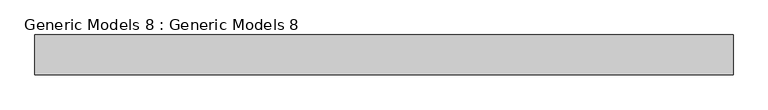
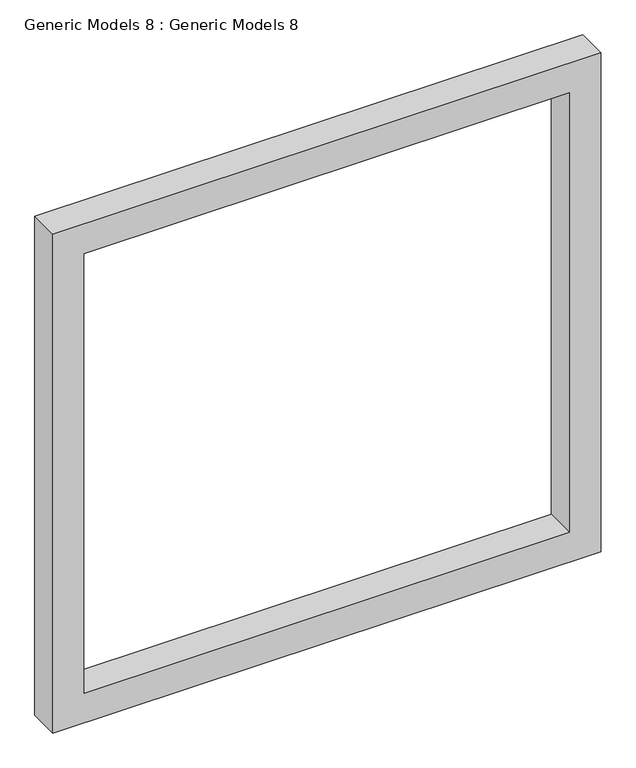
"""IFC4 building model written with IfcOpenShell, lengths in millimetres: proxy geometry, Generic Models 8 : Generic Models 8."""

from ifc_helpers import new_model, si_unit, frame, origin, place, context, project, spatial, polyline, outline, extrude, source, transform, mapped, element, save


def generic_models_8_generic_models_8_74760410(model_context):
    return source(origin(), model_context, "Body", "SweptSolid", [
        extrude(outline(polyline([(5712.5421259, -5627.8495061), (5712.5421259, -7405.8495061), (4003.166106, -7405.8495061), (4003.166106, -5627.8495061), (5712.5421259, -5627.8495061)]), holes=[polyline([(5610.9421259, -5729.4495061), (4104.766106, -5729.4495061), (4104.766106, -7304.2495061), (5610.9421259, -7304.2495061), (5610.9421259, -5729.4495061)])]), frame((0.0, -10390.4050402, 0.0), z_axis=(0.0, 1.0, 0.0), x_axis=(0.0, 0.0, 1.0)), (0.0, 0.0, 1.0), 101.6),
    ])


if __name__ == "__main__":
    model = new_model("IFC4")
    model_context = context("Model", 3, world=origin())
    ifc_project = project(units=[si_unit("LENGTHUNIT", "METRE", prefix="MILLI")], contexts=[model_context])
    site = spatial("IfcSite", under=ifc_project)
    building = spatial("IfcBuilding", under=site)
    placement = place(None, origin())
    generic_models_8_generic_models_8_shape = generic_models_8_generic_models_8_74760410(model_context)
    element("IfcBuildingElementProxy", 1, Name="Generic Models 8 : Generic Models 8", ObjectType="Generic Models 8 : Generic Models 8", at=placement, inside=building, context=model_context, shape_type="MappedRepresentation", body=[
        mapped(generic_models_8_generic_models_8_shape, transform((0.0, 0.0, 0.0), x_axis=(1.0, 0.0, 0.0), y_axis=(0.0, 1.0, 0.0), z_axis=(0.0, 0.0, 1.0))),
    ])
    save(model, "model.ifc")

# Revit data of these elements
# Element 1 (IfcBuildingElementProxy, "Generic Models 8 : Generic Models 8")
#   Materials on its faces: "ACCENT BEIGE COLOUR"
# Materials
#   "ACCENT BEIGE COLOUR": class "Generic", colour RGB 120 120 120, transparency 0, Cost = 0
